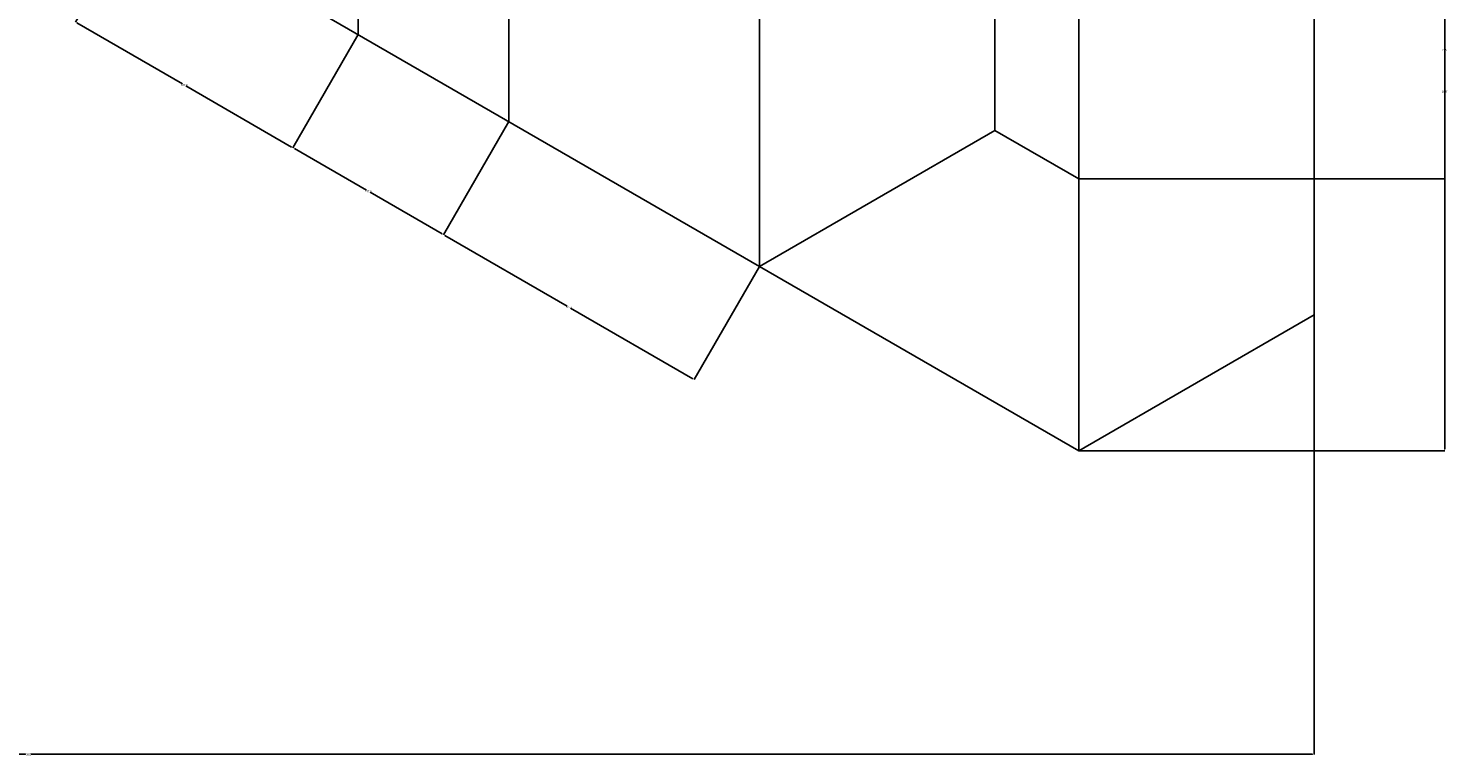
# Model space of a CAD drawing. Units: metres. Extents: x -2391 to 4922, y -635 to 4845.
# Tile 29 of 37: x 1265 to 4922, y -635 to 1238. Entities that reach past the tile are written whole.
import ezdxf

# ---------------------------------------------------------------- set-up
doc = ezdxf.new("R2010")
doc.units = ezdxf.units.M
doc.header["$MEASUREMENT"] = 0
doc.layers.add('A-ANNO-DIMS', color=2, linetype='Continuous', lineweight=18)
doc.layers.add('A-FLOR-FIXT', color=3, linetype='Continuous', lineweight=25)
doc.styles.get("Standard").update_dxf_attribs({"font": 'arial.ttf'})
doc.dimstyles.get("Standard").update_dxf_attribs({"dimtxt": 5, "dimasz": 4, "dimexe": 0.18, "dimexo": 0.0625, "dimgap": 0.09, "dimtad": 0, "dimtih": 1, "dimtoh": 1, "dimdec": 0, "dimzin": 0, "dimdsep": 46, "dimtxsty": 'Standard', "dimcen": 0.09, "dimadec": 0, "dimazin": 0, "dimtfac": 1, "dimtdec": 0, "dimtofl": 0, "dimtmove": 0, "dimatfit": 3, "dimfxl": 1, "dimtolj": 1, "dimtzin": 0, "dimarcsym": 0})

# ---------------------------------------------------------------- blocks, each defined once
blk = doc.blocks.new('*D8')
at = {"layer": 'A-ANNO-DIMS', "color": 0, "lineweight": -2, "transparency": 16777216}
for p, q in [((-2047.3, 3005.2), (-2047.3, -631.4)), ((4577.8, 2350.2), (4577.8, -631.4)), ((-2043.3, -631.2), (1257.6, -631.2)), ((4573.8, -631.2), (1272.8, -631.2))]:
    blk.add_line(p, q, dxfattribs=at)
at = {"layer": 'A-ANNO-DIMS', "color": 0, "transparency": 16777216}
for points in [[(-2043.3, -630.6), (-2043.3, -631.9), (-2047.3, -631.2)], [(4573.8, -630.6), (4573.8, -631.9), (4577.8, -631.2)]]:
    blk.add_solid(points, dxfattribs=at)
at = {"layer": 'Defpoints', "color": 0, "transparency": 16777216}
for p in [(-2047.3, 3005.3), (4577.8, 2350.3), (4577.8, -631.2)]:
    blk.add_point(p, dxfattribs=at)
at = {"layer": 'A-ANNO-DIMS', "color": 0, "transparency": 16777216, "insert": (1265.2, -631.2), "char_height": 5, "attachment_point": 5}
blk.add_mtext('\\A1;6625', dxfattribs=at)
blk = doc.blocks.new('*D20')
at = {"layer": 'A-ANNO-DIMS', "color": 0, "lineweight": -2, "transparency": 16777216}
for p, q in [((1554.6, 1545.6), (1386.3, 1254.1)), ((1389.8, 1252.3), (1662.1, 1095.1)), ((2115.2, 1222), (1946.9, 930.4)), ((1943.5, 932.6), (1671.3, 1089.8))]:
    blk.add_line(p, q, dxfattribs=at)
at = {"layer": 'A-ANNO-DIMS', "color": 0, "transparency": 16777216}
for points in [[(1390.2, 1252.8), (1389.5, 1251.7), (1386.4, 1254.3)], [(1943.9, 933.2), (1943.2, 932), (1947, 930.6)]]:
    blk.add_solid(points, dxfattribs=at)
at = {"layer": 'Defpoints', "color": 0, "transparency": 16777216}
for p in [(1554.6, 1545.7), (1386.4, 1254.3), (2115.2, 1222)]:
    blk.add_point(p, dxfattribs=at)
at = {"layer": 'A-ANNO-DIMS', "color": 0, "transparency": 16777216, "insert": (1666.7, 1092.4), "char_height": 5, "attachment_point": 5}
blk.add_mtext('\\A1;647.3', dxfattribs=at)
blk = doc.blocks.new('*D21')
at = {"layer": 'A-ANNO-DIMS', "color": 0, "lineweight": -2, "transparency": 16777216}
for p, q in [((2115.2, 1222), (1946.9, 930.4)), ((2503, 998.1), (2334.7, 706.5)), ((1950.5, 928.6), (2136.3, 821.3)), ((2331.3, 708.7), (2145.5, 816))]:
    blk.add_line(p, q, dxfattribs=at)
at = {"layer": 'A-ANNO-DIMS', "color": 0, "transparency": 16777216}
for points in [[(1950.8, 929.2), (1950.1, 928), (1947, 930.6)], [(2331.7, 709.3), (2331, 708.1), (2334.8, 706.7)]]:
    blk.add_solid(points, dxfattribs=at)
at = {"layer": 'Defpoints', "color": 0, "transparency": 16777216}
for p in [(2115.2, 1222), (2503, 998.1), (1947, 930.6)]:
    blk.add_point(p, dxfattribs=at)
at = {"layer": 'A-ANNO-DIMS', "color": 0, "transparency": 16777216, "insert": (2140.9, 818.6), "char_height": 5, "attachment_point": 5}
blk.add_mtext('\\A1;447.8', dxfattribs=at)
blk = doc.blocks.new('*D22')
at = {"layer": 'A-ANNO-DIMS', "color": 0, "lineweight": -2, "transparency": 16777216}
for p, q in [((2503, 998.1), (2334.7, 706.5)), ((2338.3, 704.7), (2653.1, 522.9)), ((3148.8, 625.2), (2980.5, 333.7)), ((2977.1, 335.9), (2662.2, 517.6))]:
    blk.add_line(p, q, dxfattribs=at)
at = {"layer": 'A-ANNO-DIMS', "color": 0, "transparency": 16777216}
for points in [[(2338.6, 705.3), (2337.9, 704.1), (2334.8, 706.7)], [(2977.4, 336.4), (2976.8, 335.3), (2980.6, 333.9)]]:
    blk.add_solid(points, dxfattribs=at)
at = {"layer": 'Defpoints', "color": 0, "transparency": 16777216}
for p in [(2503, 998.1), (2334.8, 706.7), (3148.8, 625.3)]:
    blk.add_point(p, dxfattribs=at)
at = {"layer": 'A-ANNO-DIMS', "color": 0, "transparency": 16777216, "insert": (2657.7, 520.3), "char_height": 5, "attachment_point": 5}
blk.add_mtext('\\A1;745.7', dxfattribs=at)
blk = doc.blocks.new('*D27')
at = {"layer": 'A-ANNO-DIMS', "color": 0, "lineweight": -2, "transparency": 16777216}
for p, q in [((3971.6, 2000.3), (4914.4, 2000.3)), ((4914.3, 1996.3), (4914.3, 1077.9)), ((4914.3, 154.3), (4914.3, 1072.6)), ((3971.6, 150.3), (4914.4, 150.3))]:
    blk.add_line(p, q, dxfattribs=at)
at = {"layer": 'A-ANNO-DIMS', "color": 0, "transparency": 16777216}
for points in [[(4913.6, 1996.3), (4914.9, 1996.3), (4914.3, 2000.3)], [(4913.6, 154.3), (4914.9, 154.3), (4914.3, 150.3)]]:
    blk.add_solid(points, dxfattribs=at)
at = {"layer": 'Defpoints', "color": 0, "transparency": 16777216}
for p in [(3971.5, 2000.3), (3971.5, 150.3), (4914.3, 150.3)]:
    blk.add_point(p, dxfattribs=at)
at = {"layer": 'A-ANNO-DIMS', "color": 0, "transparency": 16777216, "insert": (4914.3, 1075.3), "char_height": 5, "attachment_point": 5}
blk.add_mtext('\\A1;1850', dxfattribs=at)
blk = doc.blocks.new('*D31')
at = {"layer": 'A-ANNO-DIMS', "color": 0, "lineweight": -2, "transparency": 16777216}
for p, q in [((3971.6, 1515.3), (4914.4, 1515.3)), ((4914.3, 1511.3), (4914.3, 1185.4)), ((4914.3, 854.3), (4914.3, 1180.1)), ((3971.6, 850.3), (4914.4, 850.3))]:
    blk.add_line(p, q, dxfattribs=at)
at = {"layer": 'A-ANNO-DIMS', "color": 0, "transparency": 16777216}
for points in [[(4913.6, 1511.3), (4914.9, 1511.3), (4914.3, 1515.3)], [(4913.6, 854.3), (4914.9, 854.3), (4914.3, 850.3)]]:
    blk.add_solid(points, dxfattribs=at)
at = {"layer": 'Defpoints', "color": 0, "transparency": 16777216}
for p in [(3971.5, 1515.3), (3971.5, 850.3), (4914.3, 850.3)]:
    blk.add_point(p, dxfattribs=at)
at = {"layer": 'A-ANNO-DIMS', "color": 0, "transparency": 16777216, "insert": (4914.3, 1182.8), "char_height": 5, "attachment_point": 5}
blk.add_mtext('\\A1;665', dxfattribs=at)

msp = doc.modelspace()

# ---------------------------------------------------------------- linework, layer by layer
at = {"layer": 'A-FLOR-FIXT'}
for p, q in [((4577.76, 2350.2763), (4577.76, 500.2763)), ((3148.8181, 625.2763), (550.7419, 2125.2763)), ((2115.2362, 2044.6587), (2115.2362, 1222.0151)), ((3971.5422, 2000.2763), (3971.5422, 150.2763)), ((2503.0469, 1820.756), (2503.0469, 998.1124)), ((3755.0359, 975.2763), (3755.0359, 1640.2763)), ((3148.8181, 1505.2763), (3148.8181, 625.2763)), ((3148.8181, 625.2763), (3755.0359, 975.2763)), ((3755.0359, 975.2763), (3971.5422, 850.2763)), ((3971.5422, 150.2763), (3148.8181, 625.2763)), ((3971.5422, 150.2763), (4577.76, 500.2763))]:
    msp.add_line(p, q, dxfattribs=at)

# ---------------------------------------------------------------- dimensions: what is measured, and where the dimension line sits
at = {"layer": 'A-ANNO-DIMS'}
dim = msp.add_linear_dim(base=(4577.76, -631.2237), p1=(-2047.3343, 3005.2763), p2=(4577.76, 2350.2763), dimstyle='Standard', override={"dimdec": 0, "dimlfac": 1, "dimrnd": 0, "dimzin": 0, "dimdsep": 46, "dimlunit": 2}, dxfattribs=at)
dim.commit()
dim.dimension.update_dxf_attribs({"geometry": '*D8', "text_midpoint": (1265.2128, -631.2237)})
for base, p1, p2, angle, override, picture, middle in [((4914.26, 150.2763), (3971.5422, 2000.2763), (3971.5422, 150.2763), 90, {"dimdec": 0, "dimlfac": 1, "dimrnd": 0, "dimzin": 0, "dimdsep": 46, "dimlunit": 2}, '*D27', (4914.26, 1075.2763)), ((1386.3655, 1254.272), (2115.2362, 1222.0151), (1554.6155, 1545.6896), 150, {"dimdec": 1, "dimlfac": 1, "dimrnd": 0, "dimzin": 0, "dimdsep": 46, "dimlunit": 2}, '*D20', (1666.6758, 1092.4348)), ((4914.26, 850.2763), (3971.5422, 1515.2763), (3971.5422, 850.2763), 90, {"dimdec": 0, "dimlfac": 1, "dimrnd": 0, "dimzin": 0, "dimdsep": 46, "dimlunit": 2}, '*D31', (4914.26, 1182.7763)), ((1946.9862, 930.5975), (2503.0469, 998.1124), (2115.2362, 1222.0151), 150, {"dimdec": 1, "dimlfac": 1, "dimrnd": 0, "dimzin": 0, "dimdsep": 46, "dimlunit": 2}, '*D21', (2140.8915, 818.6462)), ((2334.7969, 706.6949), (3148.8181, 625.2763), (2503.0469, 998.1124), 150, {"dimdec": 1, "dimlfac": 1, "dimrnd": 0, "dimzin": 0, "dimdsep": 46, "dimlunit": 2}, '*D22', (2657.6825, 520.2768))]:
    dim = msp.add_linear_dim(base=base, p1=p1, p2=p2, angle=angle, dimstyle='Standard', override=override, dxfattribs=at)
    dim.commit()
    dim.dimension.update_dxf_attribs({"geometry": picture, "text_midpoint": middle})

doc.saveas('drawing.dxf')
